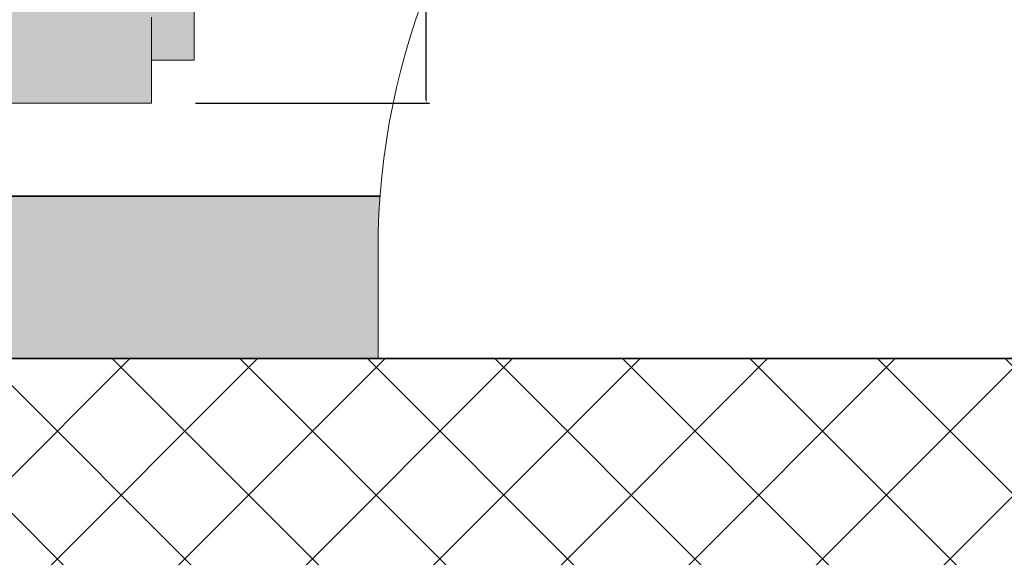
# Model space of a CAD drawing. Units: inches. Extents: x 2167 to 2589, y 1680 to 2489.
# Tile 28 of 38: x 2335 to 2389, y 1835 to 1865. Entities that reach past the tile are written whole.
import ezdxf

# ---------------------------------------------------------------- set-up
doc = ezdxf.new("R2010")
doc.units = ezdxf.units.IN
doc.header["$MEASUREMENT"] = 0
doc.layers.get('0').update_dxf_attribs({"color": 250})
for name, color, linetype, lineweight in [('A-ANNO-DIMS', 2, 'Continuous', 18), ('A-DOOR', 4, 'Continuous', 18), ('A-FURN-PATT', 31, 'Continuous', 13), ('A-WALL-PATT', 250, 'Continuous', 13), ('furniture', 34, 'Continuous', 18), ('L-PVMT-PATT', 252, 'Continuous', 13), ('walls', 7, 'Continuous', 35)]:
    doc.layers.add(name, color=color, linetype=linetype, lineweight=lineweight)
doc.styles.get("Standard").update_dxf_attribs({"font": 'arial.ttf'})
doc.dimstyles.get("Standard").update_dxf_attribs({"dimtxt": 7, "dimasz": 0.18, "dimexe": 0.18, "dimexo": 0.0625, "dimgap": 0.09, "dimtad": 0, "dimtih": 1, "dimtoh": 1, "dimdec": 1, "dimzin": 0, "dimdsep": 46, "dimlunit": 3, "dimtxsty": 'Standard', "dimcen": 0.09, "dimadec": 0, "dimazin": 0, "dimtfac": 1, "dimtdec": 1, "dimtofl": 0, "dimtmove": 0, "dimatfit": 3, "dimfxl": 1, "dimtolj": 1, "dimtzin": 0, "dimarcsym": 0})

# ---------------------------------------------------------------- blocks, each defined once
blk = doc.blocks.new('*U2')
for p, q in [((0, 0), (0, -6)), ((40, 0), (40, -6))]:
    blk.add_line(p, q)
blk.add_lwpolyline([(0, 0), (0, 40), (1.75, 40), (1.75, 0)], close=True)
blk.add_arc((0, 0), 40, 0, 90)
blk = doc.blocks.new('FABRIC SOFA 4S')
at = {"layer": 'furniture'}
for p, q in [((0, -51), (0, 51)), ((6, -51), (0, -51)), ((3, -54), (3, -51)), ((3, -54), (34, -54))]:
    blk.add_line(p, q, dxfattribs=at)
blk = doc.blocks.new('*D40')
at = {"layer": 'A-ANNO-DIMS', "color": 0, "lineweight": -2, "transparency": 16777216}
for p, q in [((2344.648, 1887.202), (2357.624, 1887.202)), ((2357.444, 1887.022), (2357.444, 1877.375)), ((2357.444, 1860.396), (2357.444, 1870.043)), ((2344.648, 1860.216), (2357.624, 1860.216))]:
    blk.add_line(p, q, dxfattribs=at)
at = {"layer": 'A-ANNO-DIMS', "color": 0, "transparency": 16777216}
for points in [[(2357.414, 1887.022), (2357.474, 1887.022), (2357.444, 1887.202)], [(2357.414, 1860.396), (2357.474, 1860.396), (2357.444, 1860.216)]]:
    blk.add_solid(points, dxfattribs=at)
at = {"layer": 'Defpoints', "color": 0, "transparency": 16777216}
for p in [(2344.585, 1887.202), (2357.444, 1887.202), (2344.585, 1860.216)]:
    blk.add_point(p, dxfattribs=at)
at = {"layer": 'A-ANNO-DIMS', "color": 0, "transparency": 16777216, "insert": (2357.444, 1873.709), "char_height": 7, "attachment_point": 5}
blk.add_mtext('\\A1;2\'-3"', dxfattribs=at)

msp = doc.modelspace()

# ---------------------------------------------------------------- hatches: boundary and pattern name
at = {"layer": 'A-FURN-PATT'}
h = msp.add_hatch(color=256, dxfattribs=at)
h.dxf.hatch_style = 1
h.paths.add_polyline_path([(2263.924, 1886.408), (2263.924, 1869.74), (2282.825, 1869.74), (2282.825, 1886.408)])
h.paths.add_polyline_path([(2282.825, 1886.408), (2282.825, 1869.74), (2301.725, 1869.74), (2301.725, 1886.408)])
h.paths.add_polyline_path([(2301.725, 1886.408), (2301.725, 1869.74), (2320.625, 1869.74), (2320.625, 1886.408)])
h.paths.add_polyline_path([(2320.625, 1886.408), (2320.625, 1869.74), (2339.525, 1869.74), (2339.525, 1886.408)])
h.paths.add_polyline_path([(2263.924, 1869.74), (2261.245, 1864.978), (2342.204, 1864.978), (2339.525, 1869.74)])
h.paths.add_polyline_path([(2261.245, 1864.978), (2261.245, 1860.216), (2342.204, 1860.216), (2342.204, 1864.978)])
h.paths.add_polyline_path([(2258.864, 1887.202), (2258.864, 1862.597), (2261.245, 1862.597), (2261.245, 1864.978), (2263.627, 1869.211), (2263.627, 1887.202)])
h.paths.add_polyline_path([(2339.823, 1887.202), (2339.823, 1869.211), (2342.204, 1864.978), (2342.204, 1862.597), (2344.585, 1862.597), (2344.585, 1887.202)])
at = {"layer": 'A-WALL-PATT'}
h = msp.add_hatch(color=256, dxfattribs=at)
h.dxf.hatch_style = 1
h.paths.add_polyline_path([(2274.738, 1855.042), (2224.048, 1855.042), (2224.048, 2003.119), (2215.048, 2003.119), (2215.048, 1846.042), (2274.738, 1846.042)])
h.paths.add_polyline_path([(2354.886, 1855.042), (2330.895, 1855.042), (2330.895, 1846.042), (2354.773, 1846.042), (2354.773, 1852.042, -0.01877)])
h.paths.add_polyline_path([(2422.048, 1864.695), (2426.208, 1864.695), (2426.208, 1867.924), (2426.208, 1869.195), (2422.048, 1869.195), (2422.048, 1916.243), (2417.548, 1916.243), (2417.548, 1855.042), (2394.773, 1855.042), (2394.773, 1852.042), (2394.773, 1846.042), (2417.548, 1846.042), (2417.548, 1779.195), (2427.738, 1779.195), (2427.738, 1783.941), (2427.738, 1788.195), (2422.048, 1788.195)])
at = {"layer": 'L-PVMT-PATT'}
h = msp.add_hatch(dxfattribs=at)
h.set_pattern_fill('ANSI37', color=256, scale=40)
h.paths.add_polyline_path([(2417.548, 1783.695), (2417.548, 1846.042), (2239.361, 1846.042), (2239.361, 1687.695), (2369.843, 1687.695), (2369.843, 1696.695), (2375.607, 1696.695), (2416.107, 1696.695), (2417.548, 1696.695)])

# ---------------------------------------------------------------- linework, layer by layer
at = {"layer": 'walls'}
for p, q in [((2224.048, 1855.042), (2354.886, 1855.042)), ((2215.048, 1846.042), (2417.548, 1846.042))]:
    msp.add_line(p, q, dxfattribs=at)

# ---------------------------------------------------------------- block references
at = {"layer": 'A-DOOR', "xscale": -1}
msp.add_blockref('*U2', (2394.773, 1852.042), dxfattribs=at)
at = {"layer": 'furniture', "xscale": 0.7937147270336093, "yscale": 0.7937147270336093, "zscale": 0.7937147270336093, "rotation": 90}
msp.add_blockref('FABRIC SOFA 4S', (2301.725, 1860.216), dxfattribs=at)

# ---------------------------------------------------------------- dimensions: what is measured, and where the dimension line sits
at = {"layer": 'A-ANNO-DIMS'}
dim = msp.add_linear_dim(base=(2357.444, 1887.202), p1=(2344.585, 1860.216), p2=(2344.585, 1887.202), angle=90, dimstyle='Standard', override={"dimdec": 1, "dimlfac": 1, "dimrnd": 0, "dimzin": 1, "dimdsep": 46, "dimlunit": 4, "dimfrac": 2}, dxfattribs=at)
dim.commit()
dim.dimension.update_dxf_attribs({"geometry": '*D40', "text_midpoint": (2357.444, 1873.709)})

doc.saveas('drawing.dxf')
